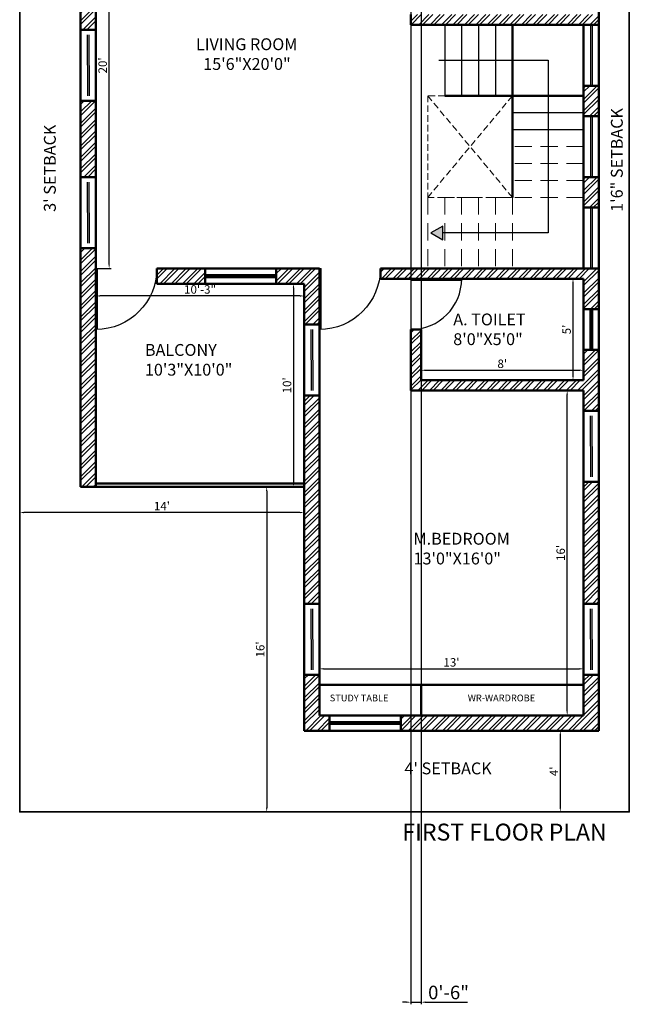
# Model space of a CAD drawing. Units: inches. Extents: x 1986 to 21484, y -1816 to 2016.
# Tile 82 of 85: x 5295 to 5655, y 953 to 1535. Entities that reach past the tile are written whole.
import ezdxf

# ---------------------------------------------------------------- set-up
doc = ezdxf.new("R2010")
doc.units = ezdxf.units.IN
doc.linetypes.add('DASHED', pattern=[19.05, 12.7, -6.35])
for name, color, linetype, lineweight in [('A-ANNO-DIMS', 2, 'Continuous', 18), ('A-ANNO-TEXT', 7, 'Continuous', 18), ('A-AREA-IDEN', 3, 'Continuous', 18), ('A-DOOR', 3, 'Continuous', 25), ('A-FLOR-STRS', 7, 'Continuous', 25), ('A-FLOR-STRS-OVHD', 8, 'DASHED', 18), ('A-GLAZ', 4, 'Continuous', 25), ('A-WALL', 7, 'Continuous', 50), ('A-WALL-PATT', 8, 'Continuous', 13), ('C-PROP', 7, 'Continuous', 35)]:
    doc.layers.add(name, color=color, linetype=linetype, lineweight=lineweight)
doc.styles.get("Standard").update_dxf_attribs({"font": 'arial.ttf'})
doc.dimstyles.new('ISO-25', dxfattribs={"dimtxt": 8, "dimasz": 2.5, "dimexe": 1.25, "dimexo": 0.625, "dimtad": 1, "dimdec": 1, "dimlunit": 3, "dimtxsty": 'Standard', "dimcen": 2.5, "dimadec": 0, "dimazin": 0, "dimtfac": 1, "dimtdec": 1, "dimtmove": 0, "dimatfit": 3, "dimfxl": 1, "dimarcsym": 0})

# ---------------------------------------------------------------- blocks, each defined once
blk = doc.blocks.new('D2')
for p, q in [((1722.5, 1505.46), (1722.5, 1475.46)), ((1723.5, 1505.46), (1723.5, 1475.46)), ((1722.5, 1475.46), (1723.5, 1475.46))]:
    blk.add_line(p, q)
blk.add_arc((1722.5, 1475.46), 30, 0, 90)
blk = doc.blocks.new('D1')
for p, q in [((1805.96, 1500.36), (1805.96, 1464.36)), ((1806.96, 1500.36), (1806.96, 1464.36)), ((1805.96, 1464.36), (1806.96, 1464.36))]:
    blk.add_line(p, q)
blk.add_arc((1805.96, 1464.36), 36, 0, 90)
blk = doc.blocks.new('*D53')
at = {"layer": 'A-ANNO-DIMS', "color": 0, "lineweight": -2, "transparency": 16777216}
for p, q in [((5471.88, 1142.38), (5471.88, 1152.54)), ((5627.88, 1142.38), (5627.88, 1152.54)), ((5474.38, 1151.29), (5625.38, 1151.29))]:
    blk.add_line(p, q, dxfattribs=at)
at = {"layer": 'A-ANNO-DIMS', "color": 0, "transparency": 16777216}
for points in [[(5474.38, 1151.71), (5474.38, 1150.88), (5471.88, 1151.29)], [(5625.38, 1151.71), (5625.38, 1150.88), (5627.88, 1151.29)]]:
    blk.add_solid(points, dxfattribs=at)
at = {"layer": 'Defpoints', "color": 0, "transparency": 16777216}
for p in [(5627.88, 1151.29), (5471.88, 1141.75), (5627.88, 1141.75)]:
    blk.add_point(p, dxfattribs=at)
at = {"layer": 'A-ANNO-DIMS', "color": 0, "transparency": 16777216, "insert": (5549.88, 1154.47), "char_height": 5, "attachment_point": 5}
blk.add_mtext("13'", dxfattribs=at)
blk = doc.blocks.new('*D54')
at = {"layer": 'A-ANNO-DIMS', "color": 0, "lineweight": -2, "transparency": 16777216}
for p, q in [((5627.26, 1315.75), (5616.95, 1315.75)), ((5618.2, 1126.25), (5618.2, 1313.25)), ((5627.26, 1123.75), (5616.95, 1123.75))]:
    blk.add_line(p, q, dxfattribs=at)
at = {"layer": 'A-ANNO-DIMS', "color": 0, "transparency": 16777216}
for points in [[(5617.78, 1313.25), (5618.61, 1313.25), (5618.2, 1315.75)], [(5617.78, 1126.25), (5618.61, 1126.25), (5618.2, 1123.75)]]:
    blk.add_solid(points, dxfattribs=at)
at = {"layer": 'Defpoints', "color": 0, "transparency": 16777216}
for p in [(5618.2, 1315.75), (5627.88, 1315.75), (5627.88, 1123.75)]:
    blk.add_point(p, dxfattribs=at)
at = {"layer": 'A-ANNO-DIMS', "color": 0, "transparency": 16777216, "insert": (5615.02, 1219.75), "char_height": 5, "attachment_point": 5, "rotation": 90}
blk.add_mtext("16'", dxfattribs=at)
blk = doc.blocks.new('*D55')
at = {"layer": 'A-ANNO-DIMS', "color": 0, "lineweight": -2, "transparency": 16777216}
for p, q in [((5531.88, 1322.38), (5531.88, 1328.91)), ((5534.38, 1327.66), (5625.38, 1327.66)), ((5627.88, 1322.38), (5627.88, 1328.91))]:
    blk.add_line(p, q, dxfattribs=at)
at = {"layer": 'A-ANNO-DIMS', "color": 0, "transparency": 16777216}
for points in [[(5534.38, 1328.08), (5534.38, 1327.25), (5531.88, 1327.66)], [(5625.38, 1328.08), (5625.38, 1327.25), (5627.88, 1327.66)]]:
    blk.add_solid(points, dxfattribs=at)
at = {"layer": 'Defpoints', "color": 0, "transparency": 16777216}
for p in [(5627.88, 1327.66), (5531.88, 1321.75), (5627.88, 1321.75)]:
    blk.add_point(p, dxfattribs=at)
at = {"layer": 'A-ANNO-DIMS', "color": 0, "transparency": 16777216, "insert": (5579.88, 1330.84), "char_height": 5, "attachment_point": 5}
blk.add_mtext("8'", dxfattribs=at)
blk = doc.blocks.new('*D56')
at = {"layer": 'A-ANNO-DIMS', "color": 0, "lineweight": -2, "transparency": 16777216}
for p, q in [((5627.26, 1381.75), (5620.39, 1381.75)), ((5621.64, 1324.25), (5621.64, 1379.25)), ((5627.26, 1321.75), (5620.39, 1321.75))]:
    blk.add_line(p, q, dxfattribs=at)
at = {"layer": 'A-ANNO-DIMS', "color": 0, "transparency": 16777216}
for points in [[(5621.23, 1379.25), (5622.06, 1379.25), (5621.64, 1381.75)], [(5621.23, 1324.25), (5622.06, 1324.25), (5621.64, 1321.75)]]:
    blk.add_solid(points, dxfattribs=at)
at = {"layer": 'Defpoints', "color": 0, "transparency": 16777216}
for p in [(5621.64, 1381.75), (5627.88, 1381.75), (5627.88, 1321.75)]:
    blk.add_point(p, dxfattribs=at)
at = {"layer": 'A-ANNO-DIMS', "color": 0, "transparency": 16777216, "insert": (5618.47, 1351.75), "char_height": 5, "attachment_point": 5, "rotation": 90}
blk.add_mtext("5'", dxfattribs=at)
blk = doc.blocks.new('*D57')
at = {"layer": 'A-ANNO-DIMS', "color": 0, "lineweight": -2, "transparency": 16777216}
for p, q in [((5462.26, 1378.75), (5455.33, 1378.75)), ((5456.58, 1376.25), (5456.58, 1261.25)), ((5462.26, 1258.75), (5455.33, 1258.75))]:
    blk.add_line(p, q, dxfattribs=at)
at = {"layer": 'A-ANNO-DIMS', "color": 0, "transparency": 16777216}
for points in [[(5456.16, 1376.25), (5457, 1376.25), (5456.58, 1378.75)], [(5456.16, 1261.25), (5457, 1261.25), (5456.58, 1258.75)]]:
    blk.add_solid(points, dxfattribs=at)
at = {"layer": 'Defpoints', "color": 0, "transparency": 16777216}
for p in [(5462.88, 1378.75), (5456.58, 1258.75), (5462.88, 1258.75)]:
    blk.add_point(p, dxfattribs=at)
at = {"layer": 'A-ANNO-DIMS', "color": 0, "transparency": 16777216, "insert": (5453.4, 1318.75), "char_height": 5, "attachment_point": 5, "rotation": 90}
blk.add_mtext("10'", dxfattribs=at)
blk = doc.blocks.new('*D58')
at = {"layer": 'A-ANNO-DIMS', "color": 0, "lineweight": -2, "transparency": 16777216}
for p, q in [((5339.88, 1378.13), (5339.88, 1370.31)), ((5462.88, 1378.13), (5462.88, 1370.31)), ((5460.38, 1371.56), (5342.38, 1371.56))]:
    blk.add_line(p, q, dxfattribs=at)
at = {"layer": 'A-ANNO-DIMS', "color": 0, "transparency": 16777216}
for points in [[(5342.38, 1371.98), (5342.38, 1371.14), (5339.88, 1371.56)], [(5460.38, 1371.98), (5460.38, 1371.14), (5462.88, 1371.56)]]:
    blk.add_solid(points, dxfattribs=at)
at = {"layer": 'Defpoints', "color": 0, "transparency": 16777216}
for p in [(5339.88, 1378.75), (5462.88, 1378.75), (5339.88, 1371.56)]:
    blk.add_point(p, dxfattribs=at)
at = {"layer": 'A-ANNO-DIMS', "color": 0, "transparency": 16777216, "insert": (5401.38, 1374.74), "char_height": 5, "attachment_point": 5}
blk.add_mtext('10\'-3"', dxfattribs=at)
blk = doc.blocks.new('*D59')
at = {"layer": 'A-ANNO-DIMS', "color": 0, "lineweight": -2, "transparency": 16777216}
for p, q in [((5340.51, 1627.75), (5348.95, 1627.75)), ((5347.7, 1390.25), (5347.7, 1625.25)), ((5340.51, 1387.75), (5348.95, 1387.75))]:
    blk.add_line(p, q, dxfattribs=at)
at = {"layer": 'A-ANNO-DIMS', "color": 0, "transparency": 16777216}
for points in [[(5347.28, 1625.25), (5348.11, 1625.25), (5347.7, 1627.75)], [(5347.28, 1390.25), (5348.11, 1390.25), (5347.7, 1387.75)]]:
    blk.add_solid(points, dxfattribs=at)
at = {"layer": 'Defpoints', "color": 0, "transparency": 16777216}
for p in [(5339.88, 1627.75), (5347.7, 1627.75), (5339.88, 1387.75)]:
    blk.add_point(p, dxfattribs=at)
at = {"layer": 'A-ANNO-DIMS', "color": 0, "transparency": 16777216, "insert": (5344.52, 1507.75), "char_height": 5, "attachment_point": 5, "rotation": 90}
blk.add_mtext("20'", dxfattribs=at)
blk = doc.blocks.new('*D72')
at = {"layer": 'A-ANNO-DIMS', "color": 0, "lineweight": -2, "transparency": 16777216}
for p, q in [((5614.14, 1112.25), (5614.14, 1069.25)), ((5614.77, 1114.75), (5615.39, 1114.75)), ((5614.77, 1066.75), (5615.39, 1066.75))]:
    blk.add_line(p, q, dxfattribs=at)
at = {"layer": 'A-ANNO-DIMS', "color": 0, "transparency": 16777216}
for points in [[(5613.72, 1112.25), (5614.56, 1112.25), (5614.14, 1114.75)], [(5613.72, 1069.25), (5614.56, 1069.25), (5614.14, 1066.75)]]:
    blk.add_solid(points, dxfattribs=at)
at = {"layer": 'Defpoints', "color": 0, "transparency": 16777216}
for p in [(5614.14, 1114.75), (5614.14, 1066.75), (5614.14, 1066.75)]:
    blk.add_point(p, dxfattribs=at)
at = {"layer": 'A-ANNO-DIMS', "color": 0, "transparency": 16777216, "insert": (5611.02, 1090.75), "char_height": 5, "attachment_point": 5, "rotation": 90}
blk.add_mtext("4'", dxfattribs=at)
blk = doc.blocks.new('*D73')
at = {"layer": 'A-ANNO-DIMS', "color": 0, "lineweight": -2, "transparency": 16777216}
for p, q in [((5441.37, 1258.75), (5442, 1258.75)), ((5440.75, 1256.25), (5440.75, 1069.25)), ((5441.37, 1066.75), (5442, 1066.75))]:
    blk.add_line(p, q, dxfattribs=at)
at = {"layer": 'A-ANNO-DIMS', "color": 0, "transparency": 16777216}
for points in [[(5440.33, 1256.25), (5441.17, 1256.25), (5440.75, 1258.75)], [(5440.33, 1069.25), (5441.17, 1069.25), (5440.75, 1066.75)]]:
    blk.add_solid(points, dxfattribs=at)
at = {"layer": 'Defpoints', "color": 0, "transparency": 16777216}
for p in [(5440.75, 1258.75), (5440.75, 1066.75), (5440.75, 1066.75)]:
    blk.add_point(p, dxfattribs=at)
at = {"layer": 'A-ANNO-DIMS', "color": 0, "transparency": 16777216, "insert": (5437.57, 1162.75), "char_height": 5, "attachment_point": 5, "rotation": 90}
blk.add_mtext("16'", dxfattribs=at)
blk = doc.blocks.new('*D74')
at = {"layer": 'A-ANNO-DIMS', "color": 0, "lineweight": -2, "transparency": 16777216}
for p, q in [((5294.88, 1244.24), (5294.88, 1244.86)), ((5462.88, 1244.24), (5462.88, 1244.86)), ((5460.38, 1243.61), (5297.38, 1243.61))]:
    blk.add_line(p, q, dxfattribs=at)
at = {"layer": 'A-ANNO-DIMS', "color": 0, "transparency": 16777216}
for points in [[(5297.38, 1244.03), (5297.38, 1243.2), (5294.88, 1243.61)], [(5460.38, 1244.03), (5460.38, 1243.2), (5462.88, 1243.61)]]:
    blk.add_solid(points, dxfattribs=at)
at = {"layer": 'Defpoints', "color": 0, "transparency": 16777216}
for p in [(5294.88, 1243.61), (5294.88, 1243.61), (5462.88, 1243.61)]:
    blk.add_point(p, dxfattribs=at)
at = {"layer": 'A-ANNO-DIMS', "color": 0, "transparency": 16777216, "insert": (5378.88, 1246.75), "char_height": 5, "attachment_point": 5}
blk.add_mtext("14'", dxfattribs=at)
blk = doc.blocks.new('WIN-36')
for p, q in [((0, 36), (0, 0)), ((0, 36), (0, 0)), ((1, 36), (1, 0))]:
    blk.add_line(p, q)
blk = doc.blocks.new('*D134')
at = {"layer": 'A-ANNO-DIMS', "color": 0, "lineweight": -2, "transparency": 16777216}
for p, q in [((5525.88, 1573.13), (5525.88, 953.11)), ((5531.88, 1573.13), (5531.88, 953.11)), ((5523.38, 954.36), (5520.88, 954.36)), ((5525.88, 954.36), (5531.88, 954.36)), ((5534.38, 954.36), (5559.4, 954.36))]:
    blk.add_line(p, q, dxfattribs=at)
at = {"layer": 'A-ANNO-DIMS', "color": 0, "transparency": 16777216}
for points in [[(5523.38, 954.78), (5523.38, 953.95), (5525.88, 954.36)], [(5534.38, 954.78), (5534.38, 953.95), (5531.88, 954.36)]]:
    blk.add_solid(points, dxfattribs=at)
at = {"layer": 'Defpoints', "color": 0, "transparency": 16777216}
for p in [(5525.88, 1573.75), (5531.88, 1573.75), (5531.88, 954.36)]:
    blk.add_point(p, dxfattribs=at)
at = {"layer": 'A-ANNO-DIMS', "color": 0, "transparency": 16777216, "insert": (5548.14, 959.07), "char_height": 8, "attachment_point": 5}
blk.add_mtext('0\'-6"', dxfattribs=at)

msp = doc.modelspace()

# ---------------------------------------------------------------- hatches: boundary and pattern name
at = {"layer": 'A-FLOR-STRS'}
h = msp.add_hatch(color=256, dxfattribs=at)
h.dxf.hatch_style = 1
h.paths.add_polyline_path([(5537.72, 1408.75), (5544.68, 1404.74), (5544.68, 1412.77)])
at = {"layer": 'A-WALL-PATT'}
h = msp.add_hatch(dxfattribs=at)
h.set_pattern_fill('ANSI32', color=256, scale=0.5)
h.set_pattern_definition([(45, (1297.9813, 0), (-3.367596, 3.367596), []), (45, (1300.2263, 0), (-3.367596, 3.367596), [])])
h.paths.add_polyline_path([(5459.88, 1852.75), (5330.88, 1852.75), (5330.88, 1765.75), (5339.88, 1765.75), (5339.88, 1843.75), (5459.88, 1843.75)])
h.paths.add_polyline_path([(5435.88, 1699.75), (5339.88, 1699.75), (5339.88, 1723.75), (5330.88, 1723.75), (5330.88, 1675.75), (5339.88, 1675.75), (5339.88, 1693.75), (5423.88, 1693.75), (5423.88, 1681.75), (5429.88, 1681.75), (5429.88, 1693.75), (5435.88, 1693.75)])
h.paths.add_polyline_path([(5531.88, 1852.75), (5501.88, 1852.75), (5501.88, 1843.75), (5525.88, 1843.75), (5525.88, 1573.75), (5531.88, 1573.75)])
h.paths.add_polyline_path([(5339.88, 1651.75), (5330.88, 1651.75), (5330.88, 1615.75), (5339.88, 1615.75), (5339.88, 1627.75), (5489.88, 1627.75), (5489.88, 1699.75), (5465.88, 1699.75), (5465.88, 1693.75), (5483.88, 1693.75), (5483.88, 1633.75), (5429.88, 1633.75), (5429.88, 1651.75), (5423.88, 1651.75), (5423.88, 1633.75), (5339.88, 1633.75)])
h.paths.add_polyline_path([(5339.88, 1573.75), (5330.88, 1573.75), (5330.88, 1528.77), (5339.88, 1528.77)])
h.paths.add_polyline_path([(5339.88, 1486.77), (5330.88, 1486.77), (5330.88, 1441.75), (5339.88, 1441.75)])
h.paths.add_polyline_path([(5339.88, 1399.75), (5330.88, 1399.75), (5330.88, 1258.75), (5339.88, 1258.75)])
h.paths.add_polyline_path([(5404.38, 1387.75), (5375.88, 1387.75), (5375.88, 1378.75), (5404.38, 1378.75)])
h.paths.add_polyline_path([(5471.88, 1387.75), (5446.38, 1387.75), (5446.38, 1378.75), (5462.88, 1378.75), (5462.88, 1354.75), (5471.88, 1354.75)])
h.paths.add_polyline_path([(5636.88, 1387.75), (5627.88, 1387.75), (5507.88, 1387.75), (5507.88, 1381.75), (5627.88, 1381.75), (5627.88, 1363.75), (5636.88, 1363.75)])
h.paths.add_polyline_path([(5636.88, 1495.75), (5627.88, 1495.75), (5627.88, 1477.75), (5636.88, 1477.75)])
h.paths.add_polyline_path([(5636.88, 1537.75), (5525.88, 1537.75), (5525.88, 1531.75), (5627.88, 1531.75), (5636.88, 1531.75)])
h.paths.add_polyline_path([(5636.88, 1441.75), (5627.88, 1441.75), (5627.88, 1423.75), (5636.88, 1423.75)])
h.paths.add_polyline_path([(5636.88, 1339.75), (5627.88, 1339.75), (5627.88, 1321.75), (5531.88, 1321.75), (5531.88, 1351.75), (5525.88, 1351.75), (5525.88, 1315.75), (5627.88, 1315.75), (5627.88, 1303.75), (5636.88, 1303.75)])
h.paths.add_polyline_path([(5636.88, 1261.75), (5627.88, 1261.75), (5627.88, 1189.75), (5636.88, 1189.75)])
h.paths.add_polyline_path([(5636.88, 1147.75), (5627.88, 1147.75), (5627.88, 1123.75), (5519.88, 1123.75), (5519.88, 1114.75), (5636.88, 1114.75)])
h.paths.add_polyline_path([(5471.88, 1147.75), (5462.88, 1147.75), (5462.88, 1114.75), (5477.88, 1114.75), (5477.88, 1123.75), (5471.88, 1123.75)])
h.paths.add_polyline_path([(5471.88, 1312.75), (5462.88, 1312.75), (5462.88, 1189.75), (5471.88, 1189.75)])

# ---------------------------------------------------------------- linework, layer by layer
at = {"layer": 'A-FLOR-STRS'}
for p, q in [((5545.88, 1531.75), (5545.88, 1489.75)), ((5555.88, 1531.75), (5555.88, 1489.75)), ((5565.88, 1531.75), (5565.88, 1489.75)), ((5575.88, 1531.75), (5575.88, 1489.75)), ((5627.88, 1479.75), (5585.88, 1479.75)), ((5627.88, 1469.75), (5585.88, 1469.75))]:
    msp.add_line(p, q, dxfattribs=at)
msp.add_lwpolyline([(5542.47, 1510.75), (5606.88, 1510.75), (5606.88, 1408.75), (5544.68, 1408.75)], dxfattribs=at)
msp.add_lwpolyline([(5537.72, 1408.75), (5544.68, 1404.74), (5544.68, 1412.77)], close=True, dxfattribs=at)
at = {"layer": 'A-FLOR-STRS-OVHD', "ltscale": 0.3}
for p, q in [((5535.88, 1489.75), (5585.88, 1429.75)), ((5535.88, 1429.75), (5585.88, 1489.75))]:
    msp.add_line(p, q, dxfattribs=at)
at = {"layer": 'A-FLOR-STRS-OVHD', "ltscale": 0.8}
for p, q in [((5627.88, 1459.75), (5585.88, 1459.75)), ((5627.88, 1449.75), (5585.88, 1449.75)), ((5627.88, 1439.75), (5585.88, 1439.75)), ((5535.88, 1429.75), (5535.88, 1387.75)), ((5627.88, 1429.75), (5535.88, 1429.75)), ((5545.88, 1429.75), (5545.88, 1387.75)), ((5555.88, 1429.75), (5555.88, 1387.75)), ((5565.88, 1429.75), (5565.88, 1387.75)), ((5575.88, 1429.75), (5575.88, 1387.75)), ((5585.88, 1429.75), (5585.88, 1387.75))]:
    msp.add_line(p, q, dxfattribs=at)
at = {"layer": 'A-FLOR-STRS-OVHD', "ltscale": 0.3}
msp.add_lwpolyline([(5535.88, 1429.75), (5585.88, 1429.75), (5585.88, 1489.75), (5535.88, 1489.75)], close=True, dxfattribs=at)
at = {"layer": 'A-WALL'}
for p, q in [((5330.88, 1258.75), (5330.88, 1852.75)), ((5636.88, 1852.75), (5636.88, 1114.75)), ((5339.88, 1258.75), (5339.88, 1627.75)), ((5525.88, 1537.75), (5525.88, 1531.75)), ((5525.88, 1531.75), (5627.88, 1531.75)), ((5585.88, 1531.75), (5585.88, 1429.75)), ((5627.88, 1531.75), (5627.88, 1387.75)), ((5627.88, 1531.75), (5636.88, 1531.75)), ((5330.88, 1528.77), (5339.88, 1528.77)), ((5627.88, 1495.75), (5636.88, 1495.75)), ((5627.88, 1489.75), (5545.88, 1489.75)), ((5330.88, 1486.77), (5339.88, 1486.77)), ((5627.88, 1477.75), (5636.88, 1477.75)), ((5330.88, 1441.75), (5339.88, 1441.75)), ((5627.88, 1441.75), (5636.88, 1441.75)), ((5627.88, 1423.75), (5636.88, 1423.75)), ((5330.88, 1399.75), (5339.88, 1399.75)), ((5375.88, 1378.75), (5375.88, 1387.75)), ((5375.88, 1387.75), (5471.88, 1387.75)), ((5404.38, 1378.75), (5404.38, 1387.75)), ((5446.38, 1378.75), (5446.38, 1387.75)), ((5471.88, 1123.75), (5471.88, 1387.75)), ((5507.88, 1387.75), (5627.88, 1387.75)), ((5507.88, 1381.75), (5507.88, 1387.75)), ((5627.88, 1387.75), (5636.88, 1387.75)), ((5375.88, 1378.75), (5462.88, 1378.75)), ((5404.38, 1383.75), (5446.38, 1383.75)), ((5404.38, 1382.75), (5446.38, 1382.75)), ((5462.88, 1114.75), (5462.88, 1378.75)), ((5507.88, 1381.75), (5627.88, 1381.75)), ((5627.88, 1381.75), (5627.88, 1321.75)), ((5627.88, 1363.75), (5636.88, 1363.75)), ((5631.88, 1339.75), (5631.88, 1363.75)), ((5632.88, 1339.75), (5632.88, 1363.75)), ((5462.88, 1354.75), (5471.88, 1354.75)), ((5525.88, 1351.75), (5525.88, 1315.75)), ((5525.88, 1351.75), (5531.88, 1351.75)), ((5531.88, 1351.75), (5531.88, 1321.75)), ((5627.88, 1339.75), (5636.88, 1339.75)), ((5531.88, 1321.75), (5627.88, 1321.75)), ((5525.88, 1315.75), (5627.88, 1315.75)), ((5627.88, 1315.75), (5627.88, 1123.75)), ((5462.88, 1312.75), (5471.88, 1312.75)), ((5627.88, 1303.75), (5636.88, 1303.75)), ((5330.88, 1258.75), (5462.88, 1258.75)), ((5339.88, 1260.75), (5462.88, 1260.75)), ((5627.88, 1261.75), (5636.88, 1261.75)), ((5462.88, 1189.75), (5471.88, 1189.75)), ((5627.88, 1189.75), (5636.88, 1189.75)), ((5462.88, 1147.75), (5471.88, 1147.75)), ((5627.88, 1147.75), (5636.88, 1147.75)), ((5471.88, 1141.75), (5627.88, 1141.75)), ((5531.88, 1123.75), (5531.88, 1141.75)), ((5531.88, 1123.75), (5531.88, 1141.75)), ((5471.88, 1123.75), (5627.88, 1123.75)), ((5477.88, 1114.75), (5477.88, 1123.75)), ((5519.88, 1114.75), (5519.88, 1123.75)), ((5477.88, 1119.75), (5519.88, 1119.75)), ((5477.88, 1118.75), (5519.88, 1118.75)), ((5636.88, 1114.75), (5462.88, 1114.75))]:
    msp.add_line(p, q, dxfattribs=at)
at = {"layer": 'C-PROP'}
msp.add_lwpolyline([(5294.88, 1900.75), (5654.88, 1900.75), (5654.88, 1066.75), (5294.88, 1066.75)], close=True, dxfattribs=at)

# ---------------------------------------------------------------- block references
at = {"layer": 'A-DOOR', "xscale": -1, "rotation": 180}
for p in [(3533.92, 2852.11), (3665.92, 2852.11)]:
    msp.add_blockref('D1', p, dxfattribs=at)
at = {"layer": 'A-DOOR', "rotation": 270}
msp.add_blockref('D2', (4050.43, 3104.25), dxfattribs=at)
at = {"layer": 'A-GLAZ'}
for p in [(5631.88, 1495.75), (5631.88, 1441.75), (5631.88, 1387.75)]:
    msp.add_blockref('WIN-36', p, dxfattribs=at)
for p, rotation in [((5334.98, 1489.77), 0.3027934322048686), ((5334.98, 1402.75), 0.302793432207276), ((5466.98, 1315.75), 0.302793432207276), ((5631.98, 1264.75), 0.302793432207276), ((5466.98, 1150.75), 0.302793432207276), ((5631.98, 1150.75), 0.302793432207276)]:
    msp.add_blockref('WIN-36', p, dxfattribs=dict(at, rotation=rotation))

# ---------------------------------------------------------------- texts
at = {"layer": 'A-ANNO-TEXT', "char_height": 7, "attachment_point": 1, "rotation": 90}
for s, insert in [('{\\fTimes New Roman|b0|i0|c0|p18;1\'6" SETBACK}', (5644.02, 1421.26)), ("{\\fTimes New Roman|b0|i0|c0|p18;3' SETBACK}", (5309.19, 1421.26))]:
    msp.add_mtext_dynamic_manual_height_columns(s, width=105.6127, gutter_width=12.5, heights=[0], dxfattribs=dict(at, insert=insert))
at = {"layer": 'A-ANNO-TEXT', "attachment_point": 1}
for s, width, insert, char_height in [('{\\fTimes New Roman|b0|i0|c0|p18;STUDY TABLE}', 105.6127, (5477.99, 1136.07), 4), ('{\\fTimes New Roman|b0|i0|c0|p18;WR-WARDROBE}', 105.6127, (5559.5, 1136.07), 4), ("{\\fTimes New Roman|b0|i0|c0|p18;4' SETBACK}", 105.6127, (5522.12, 1095.97), 7), ('{\\fTimes New Roman|b0|i0|c0|p18;FIRST FLOOR PLAN}', 226.7688, (5520.86, 1059.84), 10)]:
    msp.add_mtext_dynamic_manual_height_columns(s, width=width, gutter_width=12.5, heights=[0], dxfattribs=dict(at, insert=insert, char_height=char_height))
at = {"layer": 'A-AREA-IDEN', "char_height": 7, "attachment_point": 1}
for s, width, insert in [('{\\fTimes New Roman|b0|i0|c0|p18;LIVING ROOM\\P  15\'6"X20\'0"}', 122.2228, (5398.99, 1523.75)), ('{\\fTimes New Roman|b0|i0|c0|p18;A. TOILET\\P8\'0"X5\'0"}', 105.6127, (5550.92, 1361.19)), ('{\\fTimes New Roman|b0|i0|c0|p18;BALCONY\\P10\'3"X10\'0"}', 105.6127, (5368.83, 1343.16)), ('{\\fTimes New Roman|b0|i0|c0|p18;M.BEDROOM \\P13\'0"X16\'0"}', 105.6127, (5527.45, 1231.63))]:
    msp.add_mtext_dynamic_manual_height_columns(s, width=width, gutter_width=12.5, heights=[0], dxfattribs=dict(at, insert=insert))

# ---------------------------------------------------------------- dimensions: what is measured, and where the dimension line sits
at = {"layer": 'A-ANNO-DIMS'}
for base, p1, p2, angle, picture, middle in [((5347.7, 1627.75), (5339.88, 1387.75), (5339.88, 1627.75), 90, '*D59', (5344.52, 1507.75)), ((5456.58, 1258.75), (5462.88, 1378.75), (5462.88, 1258.75), 90, '*D57', (5453.4, 1318.75)), ((5621.64, 1381.75), (5627.88, 1321.75), (5627.88, 1381.75), 270, '*D56', (5618.47, 1351.75)), ((5618.2, 1315.75), (5627.88, 1123.75), (5627.88, 1315.75), 270, '*D54', (5615.02, 1219.75)), ((5440.75, 1066.75), (5440.75, 1258.75), (5440.75, 1066.75), 90, '*D73', (5437.57, 1162.75)), ((5614.14, 1066.75), (5614.14, 1114.75), (5614.14, 1066.75), 90, '*D72', (5611.02, 1090.75))]:
    dim = msp.add_linear_dim(base=base, p1=p1, p2=p2, angle=angle, dimstyle='ISO-25', override={"dimtxt": 5, "dimclrd": 0, "dimclre": 0, "dimclrt": 0}, dxfattribs=at)
    dim.commit()
    dim.dimension.update_dxf_attribs({"geometry": picture, "text_midpoint": middle})
for base, p1, p2, override, picture, middle in [((5531.88, 954.36), (5525.88, 1573.75), (5531.88, 1573.75), {"dimdec": 1, "dimlfac": 1, "dimrnd": 0, "dimzin": 1, "dimdsep": 46, "dimlunit": 4, "dimfrac": 2}, '*D134', (5548.14, 959.07)), ((5339.88, 1371.56), (5462.88, 1378.75), (5339.88, 1378.75), {"dimtxt": 5, "dimclrd": 0, "dimclre": 0, "dimclrt": 0}, '*D58', (5401.38, 1374.74)), ((5627.88, 1327.66), (5531.88, 1321.75), (5627.88, 1321.75), {"dimtxt": 5, "dimclrd": 0, "dimclre": 0, "dimclrt": 0}, '*D55', (5579.88, 1330.84)), ((5294.88, 1243.61), (5462.88, 1243.61), (5294.88, 1243.61), {"dimtxt": 5, "dimclrd": 0, "dimclre": 0, "dimclrt": 0}, '*D74', (5378.88, 1246.75)), ((5627.88, 1151.29), (5471.88, 1141.75), (5627.88, 1141.75), {"dimtxt": 5, "dimclrd": 0, "dimclre": 0, "dimclrt": 0}, '*D53', (5549.88, 1154.47))]:
    dim = msp.add_linear_dim(base=base, p1=p1, p2=p2, dimstyle='ISO-25', override=override, dxfattribs=at)
    dim.commit()
    dim.dimension.update_dxf_attribs({"geometry": picture, "text_midpoint": middle})

doc.saveas('drawing.dxf')
